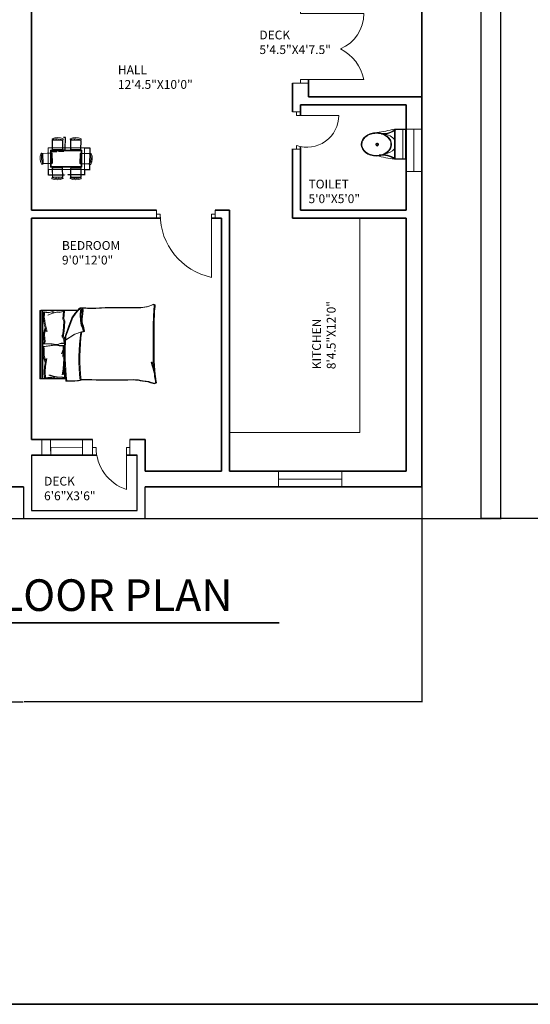
# Model space of a CAD drawing. Units: inches. Extents: x 2250 to 3629, y 982 to 2740.
# Tile 2 of 12: x 2628 to 2918, y 982 to 1543. Entities that reach past the tile are written whole.
import ezdxf

# ---------------------------------------------------------------- set-up
doc = ezdxf.new("R2010")
doc.units = ezdxf.units.IN
for name, color, linetype, lineweight in [('A-ANNO-DIMS', 2, 'Continuous', 18), ('A-ANNO-TITL', 7, 'Continuous', 35), ('A-ANNO-TTLB', 7, 'Continuous', 35), ('A-AREA-IDEN', 7, 'Continuous', 18), ('A-DOOR', 3, 'Continuous', 18), ('A-FLOR-DECK', 7, 'Continuous', 25), ('A-FLOR-FIXT', 9, 'Continuous', 18), ('A-FURN', 8, 'Continuous', 13), ('A-GLAZ', 4, 'Continuous', 18), ('A-WALL', 7, 'Continuous', 35)]:
    doc.layers.add(name, color=color, linetype=linetype, lineweight=lineweight)
doc.styles.get("Standard").update_dxf_attribs({"font": 'arial.ttf'})
doc.dimstyles.get("Standard").update_dxf_attribs({"dimtxt": 0.18, "dimasz": 0.18, "dimexe": 0.18, "dimexo": 0.0625, "dimgap": 0.09, "dimtad": 0, "dimtih": 1, "dimtoh": 1, "dimdec": 4, "dimzin": 0, "dimdsep": 46, "dimtxsty": 'Standard', "dimcen": 0.09, "dimadec": 0, "dimazin": 0, "dimtfac": 1, "dimtdec": 4, "dimtofl": 0, "dimtmove": 0, "dimatfit": 3, "dimfxl": 1, "dimtolj": 1, "dimtzin": 0, "dimarcsym": 0})

# ---------------------------------------------------------------- blocks, each defined once
blk = doc.blocks.new('A$C31115884')
for p, q in [((258, 466), (258, 523)), ((283, 498), (223, 498)), ((0, 200), (0, 0)), ((520, 200), (0, 200)), ((10, 190), (10, 10)), ((510, 190), (10, 190)), ((510, 10), (510, 190)), ((520, 0), (520, 200)), ((510, 54), (0, 54)), ((10, 10), (510, 10)), ((0, 0), (520, 0))]:
    blk.add_line(p, q)
blk.add_circle((256, 496), 23.6)
for centre, radius, start, end in [((2778, -205), 2807, 165.4549, 171.7133), ((-295, 403), 365, 324.2091, 9.3499), ((-295, 403), 375, 324.2091, 9.3499), ((384, 406), 293, 190.2774, 224.1564), ((139, 406), 293, 315.8436, 2.6563), ((806, 403), 375, 179.2036, 215.7909), ((806, 403), 365, 170.6501, 215.7909), ((3237, 905), 2807, 188.2867, 194.5451)]:
    blk.add_arc(centre, radius, start, end)
blk.add_ellipse((256, 510), major_axis=(0, -261), ratio=0.772727)
blk.add_open_spline([(256, 259), (263, 259), (270, 260), (288, 262), (299, 265), (320, 273), (330, 278), (350, 291), (360, 299), (378, 316), (386, 326), (402, 347), (409, 358), (421, 383), (427, 395), (436, 422), (440, 436), (445, 465), (447, 480), (448, 509), (448, 524), (445, 553), (443, 568), (436, 596), (432, 610), (422, 636), (416, 649), (402, 672), (395, 683), (379, 703), (370, 712), (351, 728), (341, 735), (321, 746), (310, 751), (289, 757), (278, 759), (256, 761), (245, 761), (223, 757), (212, 754), (191, 746), (181, 741), (161, 728), (151, 720), (133, 703), (125, 693), (110, 672), (103, 660), (90, 636), (85, 623), (76, 596), (72, 582), (67, 553), (66, 538), (64, 509), (65, 494), (68, 465), (70, 450), (77, 422), (81, 408), (91, 382), (97, 370), (111, 346), (118, 335), (135, 316), (144, 307), (162, 291), (172, 284), (193, 273), (203, 269), (225, 262), (236, 260), (250, 259), (253, 259), (256, 259)], degree=3, knots=[0, 0, 0, 0, 0.110105, 0.110105, 0.285049, 0.285049, 0.459994, 0.459994, 0.634938, 0.634938, 0.809882, 0.809882, 0.984827, 0.984827, 1.159771, 1.159771, 1.334715, 1.334715, 1.50966, 1.50966, 1.684604, 1.684604, 1.859549, 1.859549, 2.034493, 2.034493, 2.209437, 2.209437, 2.384382, 2.384382, 2.559326, 2.559326, 2.73427, 2.73427, 2.909215, 2.909215, 3.084159, 3.084159, 3.259103, 3.259103, 3.434048, 3.434048, 3.608992, 3.608992, 3.783936, 3.783936, 3.958881, 3.958881, 4.133825, 4.133825, 4.30877, 4.30877, 4.483714, 4.483714, 4.658658, 4.658658, 4.833603, 4.833603, 5.008547, 5.008547, 5.183491, 5.183491, 5.358436, 5.358436, 5.53338, 5.53338, 5.708324, 5.708324, 5.883269, 5.883269, 6.058213, 6.058213, 6.233158, 6.233158, 6.283185, 6.283185, 6.283185, 6.283185])
blk = doc.blocks.new('DR-72-DECK-EAST-S')
for p, q in [((5.33, 41.58), (0, 41.58)), ((0, 41.58), (4.45, 41.58)), ((9, 41.58), (1.67, 41.58)), ((1.67, 41.58), (5.33, 41.58)), ((4.45, 41.58), (4.45, 39.58)), ((4.45, 39.58), (40.45, 39.58)), ((4.5, 0), (4.5, 2)), ((4.5, 2), (40.5, 2)), ((9, 0), (0, 0)), ((0, 0), (4.5, 0))]:
    blk.add_line(p, q)
for centre, radius, start, end in [((18.64, 39.58), 21.82, 293.079, 0), ((16.02, -2.8), 24.94, 11.0871, 63.4091)]:
    blk.add_arc(centre, radius, start, end)
blk = doc.blocks.new('DR-24-BATH-SE')
for p, q in [((4.5, 21.1), (0, 21.1)), ((0, 21.1), (2.25, 21.1)), ((2.25, 21.1), (2.25, 19.1)), ((2.25, 19.1), (26.25, 19.1)), ((4.5, 0), (0, 0)), ((0, 0), (2.25, 0)), ((2.25, 0), (2.25, 2))]:
    blk.add_line(p, q)
blk.add_arc((8.16, 19.1), 18.09, 250.9415, 0)
blk = doc.blocks.new('DR-36-BED-SE')
for p, q in [((0, 38.25), (0, 33.75)), ((0, 33.75), (0, 36)), ((0, 36), (2, 36)), ((33.26, 36), (31.26, 36)), ((31.26, 36), (31.26, 0)), ((33.26, 33.75), (33.26, 38.25)), ((33.26, 38.25), (33.26, 36))]:
    blk.add_line(p, q)
blk.add_arc((38.78, 36), 36.78, 180, 258.2131)
blk = doc.blocks.new('DR-24-DECK-SE')
for p, q in [((0, 28.5), (0, 19.5)), ((21.23, 19.5), (21.23, 28.5)), ((0, 19.5), (0, 24)), ((0, 24), (2, 24)), ((21.23, 24), (19.23, 24)), ((19.23, 24), (19.23, 0))]:
    blk.add_line(p, q)
blk.add_arc((27.33, 24), 25.33, 180, 251.365)
blk = doc.blocks.new('WIN-24-DECK-NE')
for p, q in [((0, 4.5), (0, 9)), ((0, 9), (0, 0)), ((24, 0), (24, 9)), ((24, 9), (24, 4.5)), ((24, 4.5), (0, 4.5))]:
    blk.add_line(p, q)
blk = doc.blocks.new('WIN-18-DECK-SW')
for p, q in [((0, 9), (0, 0)), ((18.04, 4.5), (18.04, 9)), ((18.04, 9), (18.04, 0)), ((0, 0), (0, 4.5)), ((0, 4.5), (18.04, 4.5))]:
    blk.add_line(p, q)
blk = doc.blocks.new('WIN-36-KITCHEN-SE')
for p, q in [((0, 9), (0, 0)), ((36, 4.5), (36, 9)), ((36, 9), (36, 0)), ((0, 0), (0, 4.5)), ((0, 4.5), (36, 4.5))]:
    blk.add_line(p, q)
blk = doc.blocks.new('BED-WITH-PILLOWS')
for p, q in [((2.83, 51.56), (2.83, 66.3)), ((2.83, 66.3), (41.74, 66.3)), ((2.83, 65.05), (41.74, 65.05)), ((3.02, 51.04), (3.02, 65.78)), ((3.02, 65.78), (41.92, 65.78)), ((3.02, 64.53), (41.92, 64.53)), ((3.17, 63.59), (6.66, 63.85)), ((3.17, 63.6), (3.64, 61.01)), ((3.36, 63.06), (6.85, 63.33)), ((3.36, 63.08), (3.83, 60.49)), ((6.66, 63.85), (6.75, 63.84)), ((6.75, 63.84), (9.86, 63.6)), ((6.85, 63.33), (6.93, 63.32)), ((6.93, 63.32), (10.04, 63.08)), ((9.86, 63.6), (14.33, 62.78)), ((10.04, 63.08), (14.52, 62.26)), ((12.09, 63.25), (13.74, 63.84)), ((12.28, 62.73), (13.93, 63.32)), ((13.74, 63.84), (16.09, 64.43)), ((13.93, 63.32), (16.28, 63.91)), ((16.09, 64.43), (16.36, 64.43)), ((16.28, 63.91), (16.54, 63.91)), ((16.36, 64.43), (19.98, 64.31)), ((16.54, 63.91), (20.16, 63.79)), ((19.98, 64.31), (21.15, 64.78)), ((20.16, 63.79), (21.34, 64.26)), ((21.15, 64.78), (21.62, 60.43)), ((21.34, 64.26), (21.81, 59.9)), ((22.78, 64.27), (22.58, 59.9)), ((22.96, 63.75), (22.76, 59.38)), ((23.98, 63.88), (22.78, 64.27)), ((24.17, 63.36), (22.96, 63.75)), ((27.59, 64.22), (23.98, 63.88)), ((27.77, 63.7), (24.17, 63.36)), ((27.85, 64.24), (27.59, 64.22)), ((28.03, 63.72), (27.77, 63.7)), ((30.23, 63.8), (27.85, 64.24)), ((30.42, 63.28), (28.03, 63.72)), ((34.12, 63.8), (29.71, 62.7)), ((34.31, 63.28), (29.9, 62.18)), ((31.91, 63.31), (30.23, 63.8)), ((32.1, 62.79), (30.42, 63.28)), ((37.22, 64.23), (34.12, 63.8)), ((37.4, 63.71), (34.31, 63.28)), ((40.8, 64.22), (36.4, 64.3)), ((36.4, 64.3), (37.22, 64.23)), ((40.98, 63.7), (36.58, 63.78)), ((36.58, 63.78), (37.4, 63.71)), ((40.14, 59.58), (39.18, 61.76)), ((40.8, 64.22), (40.49, 61.61)), ((40.98, 63.7), (40.67, 61.09)), ((41.74, 66.3), (41.74, 44.64)), ((41.92, 65.78), (41.92, 44.12)), ((3.64, 61.01), (3.29, 58.89)), ((3.29, 58.89), (3.76, 58.07)), ((3.83, 60.49), (3.47, 58.37)), ((3.47, 58.37), (3.95, 57.55)), ((3.64, 56.07), (4.11, 59.01)), ((3.88, 54.78), (3.64, 56.07)), ((3.83, 55.55), (4.3, 58.49)), ((4.11, 59.01), (4.94, 61.25)), ((4.3, 58.49), (5.12, 60.73)), ((21.62, 60.43), (22.09, 57.84)), ((22.09, 56.78), (21.62, 55.25)), ((21.81, 59.9), (22.28, 57.32)), ((22.28, 56.26), (21.81, 54.73)), ((22.09, 57.84), (22.09, 56.78)), ((22.58, 59.9), (22.27, 57.28)), ((22.27, 57.28), (22.34, 56.23)), ((22.28, 57.32), (22.28, 56.26)), ((22.34, 56.23), (22.9, 54.73)), ((22.76, 59.38), (22.46, 56.76)), ((22.46, 56.76), (22.52, 55.71)), ((40.33, 59.06), (39.37, 61.24)), ((40.8, 56.67), (40.14, 59.58)), ((40.98, 56.15), (40.33, 59.06)), ((40.49, 61.61), (40.97, 59.51)), ((40.97, 59.51), (40.55, 58.66)), ((40.64, 55.37), (40.8, 56.67)), ((40.67, 61.09), (41.16, 58.99)), ((41.16, 58.99), (40.74, 58.14)), ((40.83, 54.85), (40.98, 56.15)), ((3.41, 52.19), (3.88, 54.78)), ((7.56, 52.77), (3.41, 52.19)), ((3.59, 51.66), (4.06, 54.25)), ((7.74, 52.25), (3.59, 51.66)), ((4.06, 54.25), (3.83, 55.55)), ((5.2, 53.58), (8.48, 53.04)), ((5.38, 53.06), (8.66, 52.52)), ((8.48, 53.04), (7.56, 52.77)), ((8.66, 52.52), (7.74, 52.25)), ((8.48, 53.04), (14.18, 52.69)), ((8.66, 52.52), (14.37, 52.17)), ((14.18, 52.69), (15.78, 53.14)), ((14.37, 52.17), (15.97, 52.62)), ((15.78, 53.14), (19.96, 52.81)), ((15.97, 52.62), (20.14, 52.29)), ((19.62, 53.06), (17.06, 53.95)), ((19.81, 52.54), (17.25, 53.43)), ((21.62, 53.06), (19.62, 53.06)), ((21.81, 52.54), (19.81, 52.54)), ((21.62, 55.25), (21.62, 53.06)), ((21.81, 54.73), (21.81, 52.54)), ((22.52, 55.71), (23.09, 54.21)), ((22.9, 54.73), (23.04, 52.55)), ((23.04, 52.55), (25.03, 52.68)), ((23.09, 54.21), (23.22, 52.03)), ((23.22, 52.03), (25.22, 52.15)), ((24.63, 52.15), (28.05, 46.86)), ((24.82, 51.63), (28.23, 46.34)), ((25.03, 52.68), (27.53, 53.72)), ((25.22, 52.15), (27.72, 53.2)), ((33.09, 49.76), (26.3, 52.15)), ((33.27, 49.24), (26.49, 51.63)), ((26.51, 53.58), (29.79, 53.04)), ((26.7, 53.06), (29.98, 52.52)), ((29.79, 53.04), (35.5, 52.69)), ((29.98, 52.52), (35.69, 52.17)), ((35.5, 52.69), (37.1, 53.14)), ((35.69, 52.17), (37.28, 52.62)), ((37.1, 53.14), (41.27, 52.81)), ((37.28, 52.62), (41.46, 52.29)), ((41.27, 52.81), (40.64, 55.37)), ((41.46, 52.29), (40.83, 54.85)), ((28.05, 46.86), (29.43, 43.21)), ((28.23, 46.34), (29.62, 42.69)), ((37.63, 48.12), (33.09, 49.76)), ((37.81, 47.6), (33.27, 49.24)), ((40.02, 46.36), (37.63, 48.12)), ((40.21, 45.84), (37.81, 47.6)), ((43.04, 43.71), (40.02, 46.36)), ((43.23, 43.19), (40.21, 45.84)), ((29.43, 43.21), (29.68, 41.57)), ((29.62, 42.69), (29.87, 41.05)), ((29.68, 41.57), (31.7, 42.08)), ((29.87, 41.05), (31.89, 41.56)), ((31.7, 42.08), (33.34, 42.83)), ((31.89, 41.56), (33.53, 42.31)), ((33.34, 42.83), (36.11, 43.21)), ((33.53, 42.31), (36.3, 42.69)), ((36.11, 43.21), (39.27, 43.46)), ((36.3, 42.69), (39.45, 42.94)), ((39.27, 43.46), (41.79, 43.21)), ((39.45, 42.94), (41.97, 42.69)), ((41.79, 43.21), (43.04, 43.71)), ((41.97, 42.69), (43.23, 43.19)), ((43.1, 42.29), (43.04, 43.71, 3.15)), ((43.29, 41.77), (43.23, 43.19, 3.15)), ((12.26, 1.79), (32.3, 1.79)), ((12.45, 1.27), (32.49, 1.27))]:
    blk.add_line(p, q)
for centre, radius, start, end in [((69.33, 49.94), 67.82, 178.7218, 185.604), ((17.39, -81.91), 134.3, 86.0865, 96.7821), ((69.52, 49.42), 67.82, 178.7218, 185.604), ((17.57, -82.43), 134.3, 86.0865, 96.7821), ((14.46, -60.96), 105.04, 81.7845, 96.9006), ((14.64, -61.48), 105.04, 81.7845, 96.9006), ((-136.21, 40.92), 138.49, 358.4762, 1.0082), ((-136.02, 40.4), 138.49, 358.4762, 1.0082), ((29.83, 41.52), 0.15, 160.2464, 271.1377), ((25.36, 65.1), 24.14, 280.6617, 289.8806), ((30.01, 41), 0.15, 160.2464, 271.1377), ((25.55, 64.58), 24.14, 280.6617, 289.8806), ((35.61, 37.76), 5.07, 78.6608, 113.7384), ((35.8, 37.23), 5.07, 78.6608, 113.7384), ((41.79, 71.72), 29.46, 259.8763, 272.5657), ((41.97, 71.2), 29.46, 259.8763, 272.5657), ((148.38, 36.74), 105.43, 176.9791, 183.8365), ((148.57, 36.22), 105.43, 176.9791, 183.8365), ((394.7, 25.1), 392.65, 178.2277, 181.7185), ((394.88, 24.58), 392.65, 178.2277, 181.7185), ((-3670.6, 11.09), 3713.84, 0.00217, 0.28689), ((-3670.41, 10.57), 3713.84, 0.00217, 0.28689), ((-21.9, 13.78), 24.13, 346.0648, 358.9113), ((-21.71, 13.26), 24.13, 346.0648, 358.9113), ((62, 10.4), 18.78, 177.4714, 206.4681), ((-17.63, 9.09), 19.18, 337.9751, 356.652), ((-17.45, 8.57), 19.18, 337.9751, 356.652), ((62.19, 9.88), 18.78, 177.4714, 206.4681), ((0.89, 1.4), 0.887, 146.1736, 293.4781), ((1.07, 0.88), 0.887, 146.1736, 293.4781), ((17.44, -97.2), 99.12, 92.9958, 99.4091), ((17.63, -97.72), 99.12, 92.9958, 99.4091), ((-14.02, 85.61), 86.67, 283.3832, 287.7053), ((-13.83, 85.09), 86.67, 283.3832, 287.7053), ((33.5, -106.51), 108.31, 84.4998, 90.6351), ((33.69, -107.03), 108.31, 84.4998, 90.6351), ((44.3, 2.09), 0.897, 242.6588, 356.02), ((44.48, 1.57), 0.897, 242.6588, 356.02)]:
    blk.add_arc(centre, radius, start, end)
blk = doc.blocks.new('CHAIR-DINING-1')
for points in [[(0.34, 5.75, -0.175809), (5.95, 5.7, 0.578392), (6.38, 6.17, 0.214524), (0.04, 6.26, 0.552014), (0.34, 5.75, -0.065079)], [(3.88, 5.52), (3.88, 6.18, -0.064759)], [(5.71, 5.52), (0.5, 5.52, 0.414214), (0.14, 5.16), (0.14, 0.36, 0.414214), (0.5, 0), (5.71, 0, 0.414214), (6.08, 0.36), (6.08, 5.16, 0.414214), (5.71, 5.52)]]:
    blk.add_lwpolyline(points, format="xyb")
blk.add_lwpolyline([(2.42, 6.19), (2.42, 5.52)])
blk.add_lwpolyline([(0.5, 5.36), (5.55, 5.36, -0.414214), (5.91, 4.99), (5.91, 0.53, -0.414214), (5.55, 0.16), (0.5, 0.16, -0.512069), (0.3, 0.53), (0.3, 4.99, -0.512069)], format="xyb", close=True)
blk = doc.blocks.new('TABLE-RECTANGULAR')
for points in [[(0, 12.37), (20.61, 12.37), (20.61, 0), (0, 0)], [(1.37, 10.99), (19.24, 10.99), (19.24, 1.37), (1.37, 1.37)], [(1.79, 10.58), (18.82, 10.58), (18.82, 1.79), (1.79, 1.79)]]:
    blk.add_lwpolyline(points, close=True)
blk = doc.blocks.new('*D63')
at = {"layer": 'A-ANNO-DIMS', "color": 0, "lineweight": -2, "transparency": 16777216}
for p, q in [((2644.02, 1457.3), (2644.02, 1454.09)), ((2664.63, 1457.3), (2664.63, 1454.09)), ((2644.2, 1454.27), (2653.36, 1454.27)), ((2664.45, 1454.27), (2655.29, 1454.27))]:
    blk.add_line(p, q, dxfattribs=at)
at = {"layer": 'A-ANNO-DIMS', "color": 0, "transparency": 16777216}
for points in [[(2644.2, 1454.3), (2644.2, 1454.24), (2644.02, 1454.27)], [(2664.45, 1454.3), (2664.45, 1454.24), (2664.63, 1454.27)]]:
    blk.add_solid(points, dxfattribs=at)
at = {"layer": 'Defpoints', "color": 0, "transparency": 16777216}
for p in [(2644.02, 1457.36), (2664.63, 1457.36), (2664.63, 1454.27)]:
    blk.add_point(p, dxfattribs=at)
at = {"layer": 'A-ANNO-DIMS', "color": 0, "transparency": 16777216, "insert": (2654.33, 1454.27), "char_height": 0.18, "attachment_point": 5}
blk.add_mtext('\\A1;TABLE 21 TYP.', dxfattribs=at)
blk = doc.blocks.new('*D64')
at = {"layer": 'A-ANNO-DIMS', "color": 0, "lineweight": -2, "transparency": 16777216}
for p, q in [((2664.69, 1469.73), (2667.9, 1469.73)), ((2667.72, 1469.55), (2667.72, 1463.73)), ((2667.72, 1457.54), (2667.72, 1463.36)), ((2664.69, 1457.36), (2667.9, 1457.36))]:
    blk.add_line(p, q, dxfattribs=at)
at = {"layer": 'A-ANNO-DIMS', "color": 0, "transparency": 16777216}
for points in [[(2667.69, 1469.55), (2667.75, 1469.55), (2667.72, 1469.73)], [(2667.69, 1457.54), (2667.75, 1457.54), (2667.72, 1457.36)]]:
    blk.add_solid(points, dxfattribs=at)
at = {"layer": 'Defpoints', "color": 0, "transparency": 16777216}
for p in [(2664.63, 1469.73), (2667.72, 1469.73), (2664.63, 1457.36)]:
    blk.add_point(p, dxfattribs=at)
at = {"layer": 'A-ANNO-DIMS', "color": 0, "transparency": 16777216, "insert": (2667.72, 1463.54), "char_height": 0.18, "attachment_point": 5}
blk.add_mtext('\\A1;12 TYP.', dxfattribs=at)
blk = doc.blocks.new('*D65')
at = {"layer": 'A-ANNO-DIMS', "color": 0, "lineweight": -2, "transparency": 16777216}
for p, q in [((2652.71, 1475.74), (2653.9, 1475.74)), ((2653.72, 1475.56), (2653.72, 1472.36)), ((2652.71, 1468.61), (2653.9, 1468.61)), ((2653.72, 1468.79), (2653.72, 1471.99))]:
    blk.add_line(p, q, dxfattribs=at)
at = {"layer": 'A-ANNO-DIMS', "color": 0, "transparency": 16777216}
for points in [[(2653.69, 1475.56), (2653.75, 1475.56), (2653.72, 1475.74)], [(2653.69, 1468.79), (2653.75, 1468.79), (2653.72, 1468.61)]]:
    blk.add_solid(points, dxfattribs=at)
at = {"layer": 'Defpoints', "color": 0, "transparency": 16777216}
for p in [(2652.65, 1475.74), (2653.72, 1475.74), (2652.65, 1468.61)]:
    blk.add_point(p, dxfattribs=at)
at = {"layer": 'A-ANNO-DIMS', "color": 0, "transparency": 16777216, "insert": (2653.72, 1472.18), "char_height": 0.18, "attachment_point": 5}
blk.add_mtext('\\A1;CHAIR A 7 TYP.', dxfattribs=at)
blk = doc.blocks.new('*D66')
at = {"layer": 'A-ANNO-DIMS', "color": 0, "lineweight": -2, "transparency": 16777216}
for p, q in [((2646.22, 1468.55), (2646.22, 1467.36)), ((2652.65, 1468.55), (2652.65, 1467.36)), ((2646.4, 1467.54), (2648.97, 1467.54)), ((2652.47, 1467.54), (2649.89, 1467.54))]:
    blk.add_line(p, q, dxfattribs=at)
at = {"layer": 'A-ANNO-DIMS', "color": 0, "transparency": 16777216}
for points in [[(2646.4, 1467.57), (2646.4, 1467.51), (2646.22, 1467.54)], [(2652.47, 1467.57), (2652.47, 1467.51), (2652.65, 1467.54)]]:
    blk.add_solid(points, dxfattribs=at)
at = {"layer": 'Defpoints', "color": 0, "transparency": 16777216}
for p in [(2646.22, 1468.61), (2652.65, 1468.61), (2652.65, 1467.54)]:
    blk.add_point(p, dxfattribs=at)
at = {"layer": 'A-ANNO-DIMS', "color": 0, "transparency": 16777216, "insert": (2649.43, 1467.54), "char_height": 0.18, "attachment_point": 5}
blk.add_mtext('\\A1;6 TYP.', dxfattribs=at)
blk = doc.blocks.new('*D169')
at = {"layer": 'A-ANNO-DIMS', "color": 0, "lineweight": -2, "transparency": 16777216}
for p, q in [((2856.61, 1276.67), (2856.61, 1154.23)), ((2403.61, 1258.67), (2403.61, 1154.23)), ((2403.79, 1154.41), (2629.81, 1154.41)), ((2856.43, 1154.41), (2630.4, 1154.41))]:
    blk.add_line(p, q, dxfattribs=at)
at = {"layer": 'A-ANNO-DIMS', "color": 0, "transparency": 16777216}
for points in [[(2403.79, 1154.44), (2403.79, 1154.38), (2403.61, 1154.41)], [(2856.43, 1154.44), (2856.43, 1154.38), (2856.61, 1154.41)]]:
    blk.add_solid(points, dxfattribs=at)
at = {"layer": 'Defpoints', "color": 0, "transparency": 16777216}
for p in [(2856.61, 1276.74), (2403.61, 1258.74), (2856.61, 1154.41)]:
    blk.add_point(p, dxfattribs=at)
at = {"layer": 'A-ANNO-DIMS', "color": 0, "transparency": 16777216, "insert": (2630.11, 1154.41), "char_height": 0.18, "attachment_point": 5}
blk.add_mtext('\\A1;453', dxfattribs=at)
blk = doc.blocks.new('*D170')
at = {"layer": 'A-ANNO-DIMS', "color": 0, "lineweight": -2, "transparency": 16777216}
for p, q in [((2855.4, 2070.24), (2901.69, 2070.24)), ((2901.51, 2070.06), (2901.51, 1664.67)), ((2901.51, 1258.92), (2901.51, 1664.3)), ((2481.67, 1258.74), (2901.69, 1258.74))]:
    blk.add_line(p, q, dxfattribs=at)
at = {"layer": 'A-ANNO-DIMS', "color": 0, "transparency": 16777216}
for points in [[(2901.48, 2070.06), (2901.54, 2070.06), (2901.51, 2070.24)], [(2901.48, 1258.92), (2901.54, 1258.92), (2901.51, 1258.74)]]:
    blk.add_solid(points, dxfattribs=at)
at = {"layer": 'Defpoints', "color": 0, "transparency": 16777216}
for p in [(2855.34, 2070.24), (2901.51, 2070.24), (2481.61, 1258.74)]:
    blk.add_point(p, dxfattribs=at)
at = {"layer": 'A-ANNO-DIMS', "color": 0, "transparency": 16777216, "insert": (2901.51, 1664.49), "char_height": 0.18, "attachment_point": 5}
blk.add_mtext('\\A1;811.5', dxfattribs=at)
blk = doc.blocks.new('*D173')
at = {"layer": 'A-ANNO-DIMS', "color": 0, "lineweight": -2, "transparency": 16777216}
for p, q in [((2932.01, 1947.92), (2890.14, 1947.92)), ((2890.32, 1947.74), (2890.32, 1603.51)), ((2890.32, 1258.92), (2890.32, 1603.15)), ((2981.16, 1258.74), (2890.14, 1258.74))]:
    blk.add_line(p, q, dxfattribs=at)
at = {"layer": 'A-ANNO-DIMS', "color": 0, "transparency": 16777216}
for points in [[(2890.29, 1947.74), (2890.35, 1947.74), (2890.32, 1947.92)], [(2890.29, 1258.92), (2890.35, 1258.92), (2890.32, 1258.74)]]:
    blk.add_solid(points, dxfattribs=at)
at = {"layer": 'Defpoints', "color": 0, "transparency": 16777216}
for p in [(2932.07, 1947.92), (2890.32, 1258.74), (2981.23, 1258.74)]:
    blk.add_point(p, dxfattribs=at)
at = {"layer": 'A-ANNO-DIMS', "color": 0, "transparency": 16777216, "insert": (2890.32, 1603.33), "char_height": 0.18, "attachment_point": 5}
blk.add_mtext('\\A1;689.2', dxfattribs=at)

msp = doc.modelspace()

# ---------------------------------------------------------------- linework, layer by layer
at = {"layer": 'A-ANNO-TITL'}
msp.add_line((2524.9884, 1199.312), (2775.3748, 1199.312), dxfattribs=at)
at = {"layer": 'A-ANNO-TTLB'}
msp.add_lwpolyline([(2249.6849, 2739.593), (3629.4532, 2739.593), (3629.4532, 982.3108), (2249.6849, 982.3108)], close=True, dxfattribs=at)
at = {"layer": 'A-FLOR-DECK'}
for p, q in [((2634.6072, 1294.7354), (2634.6072, 1276.7354)), ((2694.6258, 1263.2354), (2694.6258, 1294.7354)), ((2630.1072, 1276.7354), (2630.1072, 1258.7354)), ((2634.6072, 1276.7354), (2634.6072, 1263.2354)), ((2699.1258, 1258.7354), (2699.1258, 1276.7354)), ((2634.6072, 1263.2354), (2694.6258, 1263.2354)), ((2630.1072, 1258.7354), (2699.1258, 1258.7354))]:
    msp.add_line(p, q, dxfattribs=at)
at = {"layer": 'A-FLOR-FIXT'}
for p, q in [((2821.2796, 1429.7354), (2821.2796, 1307.7437)), ((2821.2796, 1307.7437), (2747.1072, 1307.7437))]:
    msp.add_line(p, q, dxfattribs=at)
at = {"layer": 'A-FURN'}
for points in [[(2662.3586, 1452.8277, 0.41421356), (2662.7233, 1453.1923), (2662.7233, 1457.9842, 0.41421356), (2662.3586, 1458.3489), (2657.1471, 1458.3489, 0.41421356), (2656.7824, 1457.9842), (2656.7824, 1453.1923, 0.41421356), (2657.1471, 1452.8277), (2662.3586, 1452.8277)], [(2662.5226, 1452.6024, -0.17580928), (2656.9089, 1452.6449, 0.57839206), (2656.4836, 1452.1772, 0.21452438), (2662.8203, 1452.0922, 0.55201397), (2662.5226, 1452.6024, -0.06507904)], [(2658.9776, 1452.8277), (2658.9776, 1452.1686, -0.06475861)]]:
    msp.add_lwpolyline(points, format="xyb", dxfattribs=at)
msp.add_lwpolyline([(2662.3564, 1452.9919), (2657.3113, 1452.9919, -0.41421356), (2656.9467, 1453.3565), (2656.9467, 1457.82, -0.41421356), (2657.3113, 1458.1846), (2662.3564, 1458.1846, -0.51206948), (2662.559, 1457.82), (2662.559, 1453.3565, -0.51206948)], format="xyb", close=True, dxfattribs=at)
msp.add_lwpolyline([(2660.4364, 1452.1566), (2660.4364, 1452.8277)], dxfattribs=at)
at = {"layer": 'A-GLAZ'}
for p, q in [((2640.41, 1303.7354), (2640.41, 1296.6878)), ((2640.41, 1296.6878), (2640.41, 1294.7354))]:
    msp.add_line(p, q, dxfattribs=at)
at = {"layer": 'A-WALL'}
for p, q in [((2856.6072, 2029.7354), (2856.6072, 1276.7354)), ((2634.6072, 1638.2354), (2634.6072, 1434.2354)), ((2792.1072, 1498.7354), (2792.1072, 1508.4808)), ((2783.1072, 1494.2354), (2783.1072, 1506.4808)), ((2783.1072, 1498.7354), (2783.1072, 1494.2354)), ((2792.1072, 1498.7354), (2856.6072, 1498.7354)), ((2783.1072, 1494.2354), (2783.1072, 1490.123)), ((2787.6072, 1494.2354), (2847.6072, 1494.2354)), ((2787.6072, 1488.123), (2787.6072, 1494.2354)), ((2847.6072, 1494.2354), (2847.6072, 1434.2354)), ((2783.1072, 1469.0225), (2783.1072, 1429.7354)), ((2787.6072, 1434.2354), (2787.6072, 1470.4043)), ((2634.6072, 1434.2354), (2705.7468, 1434.2354)), ((2634.6072, 1429.7354), (2634.6072, 1303.7354)), ((2707.8157, 1429.7354), (2634.6072, 1429.7354)), ((2742.6072, 1429.7354), (2737.01, 1429.7354)), ((2739.01, 1434.2354), (2747.1072, 1434.2354)), ((2742.6072, 1429.7354), (2742.6072, 1285.7354)), ((2747.1072, 1429.7354), (2747.1072, 1434.2354)), ((2747.1072, 1285.7354), (2747.1072, 1429.7354)), ((2783.1072, 1429.7354), (2847.6072, 1429.7354)), ((2783.1072, 1429.7354), (2787.6072, 1429.7354)), ((2787.6072, 1434.2354), (2847.6072, 1434.2354)), ((2847.6072, 1429.7354), (2847.6072, 1285.7354)), ((2634.6072, 1303.7354), (2669.3082, 1303.7354)), ((2690.5428, 1303.7354), (2699.1258, 1303.7354)), ((2699.1258, 1303.7354), (2699.1258, 1294.7354)), ((2671.7111, 1294.7354), (2634.6072, 1294.7354)), ((2694.6258, 1294.7354), (2688.5428, 1294.7354)), ((2699.1258, 1285.7354), (2699.1258, 1294.7354)), ((2699.1258, 1285.7354), (2742.6072, 1285.7354)), ((2847.6072, 1285.7354), (2747.1072, 1285.7354)), ((2747.1072, 1285.7354), (2847.6072, 1285.7354)), ((2481.6072, 1276.7354), (2630.1072, 1276.7354)), ((2699.1258, 1276.7354), (2856.6072, 1276.7354))]:
    msp.add_line(p, q, dxfattribs=at)

# ---------------------------------------------------------------- block references
at = {"layer": 'A-DOOR'}
for name, p in [('DR-72-DECK-EAST-S', (2783.107, 1506.481)), ('DR-24-BATH-SE', (2783.107, 1469.022)), ('DR-36-BED-SE', (2705.747, 1395.985)), ('DR-24-DECK-SE', (2669.308, 1275.235))]:
    msp.add_blockref(name, p, dxfattribs=at)
at = {"layer": 'A-FLOR-FIXT', "xscale": 0.0330640103915726, "yscale": 0.0330640103915726, "zscale": 0.0330640103915726, "rotation": 89.99999999999991}
msp.add_blockref('A$C31115884', (2847.6072, 1463.1662), dxfattribs=at)
at = {"layer": 'A-FURN'}
for name, p in [('CHAIR-DINING-1', (2646.232, 1468.608)), ('TABLE-RECTANGULAR', (2644.02, 1457.361))]:
    msp.add_blockref(name, p, dxfattribs=at)
at = {"layer": 'A-FURN', "extrusion": (0, 0, -1), "zscale": -1}
for p, rotation in [((-2662.7783, 1468.5403), 1.208770615435877), ((-2646.2536, 1466.9075), 267.467029090698)]:
    msp.add_blockref('CHAIR-DINING-1', p, dxfattribs=dict(at, rotation=rotation))
at = {"layer": 'A-FURN'}
for name, p, rotation in [('CHAIR-DINING-1', (2662.3231, 1466.743), 267.7813808549047), ('CHAIR-DINING-1', (2652.3685, 1458.4323), 181.4957379563671), ('BED-WITH-PILLOWS', (2705.6232, 1335.3633), 90.00000000000003)]:
    msp.add_blockref(name, p, dxfattribs=dict(at, rotation=rotation))
at = {"layer": 'A-GLAZ'}
for name, p, rotation in [('WIN-24-DECK-NE', (2847.6068, 1480.2354), 269.9999999999973), ('WIN-18-DECK-SW', (2645.4724, 1294.7087), 0.1672301246895337)]:
    msp.add_blockref(name, p, dxfattribs=dict(at, rotation=rotation))
msp.add_blockref('WIN-36-KITCHEN-SE', (2775.05, 1276.735), dxfattribs=at)

# ---------------------------------------------------------------- texts
at = {"layer": 'A-ANNO-TITL', "insert": (2531.7555, 1224.1419), "char_height": 18, "attachment_point": 1}
msp.add_mtext_dynamic_manual_height_columns('FIRST FLOOR PLAN', width=297.220022, gutter_width=12.5, heights=[0], dxfattribs=at)
at = {"layer": 'A-AREA-IDEN', "char_height": 5, "attachment_point": 1}
for s, width, insert in [('DECK\\P5\'4.5"X4\'7.5"', 63.091736, (2764.1841, 1536.4039)), ('HALL\\P12\'4.5"X10\'0"', 130.718243, (2683.7221, 1516.5781)), ('TOILET\\P5\'0"X5\'0"', 82.224606, (2792.1284, 1451.5585)), ('BEDROOM\\P9\'0"12\'0"', 117.579696, (2651.8883, 1416.6336)), ('DECK\\P6\'6"X3\'6"', 96.606177, (2641.7129, 1282.483))]:
    msp.add_mtext_dynamic_manual_height_columns(s, width=width, gutter_width=12.5, heights=[0], dxfattribs=dict(at, insert=insert))
at = {"layer": 'A-AREA-IDEN', "insert": (2794.2101, 1343.7121), "char_height": 5, "attachment_point": 1, "rotation": 90}
msp.add_mtext_dynamic_manual_height_columns('KITCHEN\\P8\'4.5"X12\'0"', width=145.215495, gutter_width=12.5, heights=[0], dxfattribs=at)

# ---------------------------------------------------------------- dimensions: what is measured, and where the dimension line sits
at = {"layer": 'A-ANNO-DIMS'}
for base, p1, p2, picture, middle in [((2901.5072, 2070.2354), (2481.6072, 1258.7354), (2855.3384, 2070.2354), '*D170', (2901.5072, 1664.4854)), ((2890.3241, 1258.7354), (2932.0741, 1947.9231), (2981.2267, 1258.7354), '*D173', (2890.3241, 1603.3293))]:
    dim = msp.add_linear_dim(base=base, p1=p1, p2=p2, angle=90, dimstyle='Standard', override={"dimdec": 1, "dimlfac": 1, "dimrnd": 0, "dimzin": 0, "dimdsep": 46, "dimlunit": 2}, dxfattribs=at)
    dim.commit()
    dim.dimension.update_dxf_attribs({"geometry": picture, "text_midpoint": middle})
for base, p1, p2, text, picture, middle in [((2653.7184, 1475.7438), (2652.648, 1468.6079), (2652.648, 1475.7438), 'CHAIR A <> TYP.', '*D65', (2653.7184, 1472.1759)), ((2667.7219, 1469.7278), (2664.6304, 1457.3615), (2664.6304, 1469.7278), '<> TYP.', '*D64', (2667.7219, 1463.5446))]:
    dim = msp.add_linear_dim(base=base, p1=p1, p2=p2, angle=90, text=text, dimstyle='Standard', override={"dimdec": 0, "dimlfac": 1, "dimrnd": 0, "dimzin": 0, "dimdsep": 46, "dimlunit": 2}, dxfattribs=at)
    dim.commit()
    dim.dimension.update_dxf_attribs({"geometry": picture, "text_midpoint": middle})
for base, p1, p2, text, picture, middle in [((2652.648, 1467.5376), (2646.216, 1468.6079), (2652.648, 1468.6079), '<> TYP.', '*D66', (2649.432, 1467.5376)), ((2664.6304, 1454.2699), (2644.0198, 1457.3615), (2664.6304, 1457.3615), 'TABLE <> TYP.', '*D63', (2654.3251, 1454.2699))]:
    dim = msp.add_linear_dim(base=base, p1=p1, p2=p2, text=text, dimstyle='Standard', override={"dimdec": 0, "dimlfac": 1, "dimrnd": 0, "dimzin": 0, "dimdsep": 46, "dimlunit": 2}, dxfattribs=at)
    dim.commit()
    dim.dimension.update_dxf_attribs({"geometry": picture, "text_midpoint": middle})
dim = msp.add_linear_dim(base=(2856.6072, 1154.412), p1=(2403.6072, 1258.7354), p2=(2856.6072, 1276.7354), dimstyle='Standard', override={"dimdec": 0, "dimlfac": 1, "dimrnd": 0, "dimzin": 0, "dimdsep": 46, "dimlunit": 2}, dxfattribs=at)
dim.commit()
dim.dimension.update_dxf_attribs({"geometry": '*D169', "text_midpoint": (2630.1072, 1154.412)})

doc.saveas('drawing.dxf')
